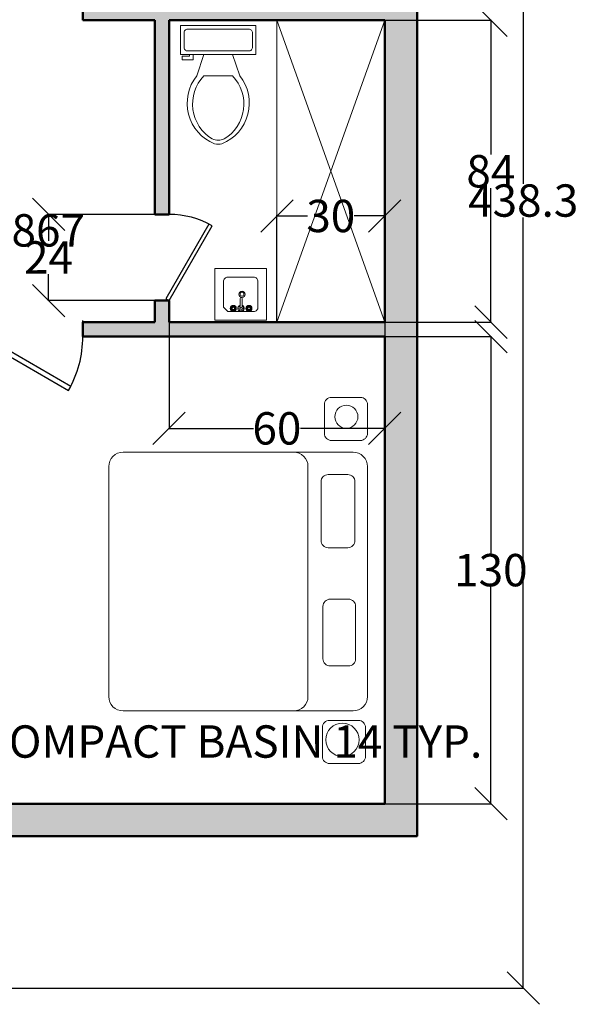
# Model space of a CAD drawing. Units: inches. Extents: x -9 to 615, y -420 to 89.
# Tile 4 of 6: x 460 to 615, y -389 to -115. Entities that reach past the tile are written whole.
import ezdxf

# ---------------------------------------------------------------- set-up
doc = ezdxf.new("R2010")
doc.units = ezdxf.units.IN
doc.header["$MEASUREMENT"] = 0
for name, color, linetype, lineweight in [('A-ANNO-DIMS', 2, 'Continuous', 18), ('A-DOOR', 4, 'Continuous', 25), ('A-FLOR-FIXT', 9, 'Continuous', 18), ('A-FURN', 8, 'Continuous', 18), ('A-WALL', 7, 'Continuous', 50)]:
    doc.layers.add(name, color=color, linetype=linetype, lineweight=lineweight)
doc.layers.add('A-WALL-PATT', color=251, linetype='Continuous', lineweight=13, true_color=0x636466)
doc.styles.get("Standard").update_dxf_attribs({"font": 'arial.ttf'})
doc.dimstyles.get("Standard").update_dxf_attribs({"dimtxt": 9, "dimasz": 9, "dimexe": 0.18, "dimexo": 0.0625, "dimgap": 0.09, "dimtad": 0, "dimtih": 1, "dimtoh": 1, "dimdec": 0, "dimzin": 0, "dimdsep": 46, "dimlunit": 4, "dimtxsty": 'Standard', "dimblk": 'OBLIQUE', "dimblk2": 'OBLIQUE', "dimcen": 0.09, "dimadec": 0, "dimazin": 0, "dimtfac": 1, "dimtdec": 0, "dimtofl": 0, "dimtmove": 0, "dimatfit": 3, "dimldrblk": 'OBLIQUE', "dimfxl": 1, "dimtolj": 1, "dimtzin": 0, "dimarcsym": 0})

# ---------------------------------------------------------------- blocks, each defined once
blk = doc.blocks.new('6 BED')
for p, q in [((-33.45, 25.64), (30.55, 25.64)), ((-37.45, 21.64), (-37.45, -23.43)), ((34.55, 21.64), (34.55, -19.64))]:
    blk.add_line(p, q)
for points in [[(-42.69, 42.2), (-50.69, 42.2, 0.414214), (-52.69, 40.2), (-52.69, 32.2, 0.414214), (-50.69, 30.2), (-42.69, 30.2, 0.414214), (-40.69, 32.2), (-40.69, 40.2, 0.414214)], [(-33.45, 42.2), (30.55, 42.2, -0.414214), (34.55, 38.2), (34.55, -25.8, -0.414214), (30.55, -29.8), (-33.45, -29.8, -0.414214), (-37.45, -25.8), (-37.45, 38.2, -0.414214)], [(39.19, 41.65), (47.19, 41.65, -0.414214), (49.19, 39.65), (49.19, 31.65, -0.414214), (47.19, 29.65), (39.19, 29.65, -0.414214), (37.19, 31.65), (37.19, 39.65, -0.414214)], [(-29.22, 38.71), (-12.85, 38.71, -0.414214), (-10.85, 36.71), (-10.85, 31.26, -0.414214), (-12.85, 29.26), (-29.22, 29.26, -0.414214), (-31.22, 31.26), (-31.22, 36.71, -0.414214)], [(5.45, 38.89), (20.03, 38.89, -0.414214), (22.03, 36.89), (22.03, 31.79, -0.414214), (20.03, 29.79), (5.45, 29.79, -0.414214), (3.45, 31.79), (3.45, 36.89, -0.414214)]]:
    blk.add_lwpolyline(points, format="xyb", close=True)
for centre, start, end in [((-33.45, 21.64), 90, 180), ((30.55, 21.64), 0, 90)]:
    blk.add_arc(centre, 4, start, end)
blk = doc.blocks.new('Toilet - top')
for p, q in [((9.5, -6), (9.5, -2)), ((-8, -8.5), (-8, -8)), ((-7, -8), (-7, -9.5)), ((-4, -8), (-6, -14)), ((4, -8), (6, -14)), ((-10, -8.5), (-8, -8.5)), ((-10, -9.5), (-10, -8.5)), ((-7, -9.5), (-10, -9.5)), ((4, -14), (-4, -14))]:
    blk.add_line(p, q)
blk.add_lwpolyline([(10.5, -8), (10.5, 0), (-10.5, 0), (-10.5, -8)], close=True)
for points in [[(-9.5, -2), (-9.5, -6)], [(8.5, -1), (-8.5, -1)], [(-8.5, -7), (8.5, -7)]]:
    blk.add_lwpolyline(points)
for centre, radius, start, end in [((-8.62, -1.88), 0.884, 81.8699, 188.1301), ((8.62, -1.88), 0.884, 351.8699, 98.1301), ((-8.62, -6.12), 0.884, 171.8699, 278.1301), ((8.62, -6.12), 0.884, 261.8699, 8.1301), ((3.52, -21.58), 12.17, 141.4691, 247.9714), ((4.2, -21.82), 11.33, 136.3677, 238.9468), ((-3.52, -21.58), 12.17, 292.0284, 38.5307), ((-4.2, -21.82), 11.33, 301.053, 43.6321), ((0, -27.88), 4, 245.7318, 294.2682), ((0, -29), 4, 254.8605, 285.1395)]:
    blk.add_arc(centre, radius, start, end)
blk = doc.blocks.new('*U12')
for p, q in [((0, 0), (0, -6)), ((40, 0), (40, -6))]:
    blk.add_line(p, q)
blk.add_lwpolyline([(0, 0), (34.64, 20), (35.52, 18.48), (0.87, -1.52)], close=True)
blk.add_arc((0, 0), 40, 0, 30)
blk = doc.blocks.new('*U13')
for p, q in [((0, 0), (0, 6)), ((40, 0), (40, 6))]:
    blk.add_line(p, q)
blk.add_lwpolyline([(0, 0), (34.64, -20), (35.52, -18.48), (0.87, 1.52)], close=True)
blk.add_arc((0, 0), 40, 330, 0)
blk = doc.blocks.new('Faucet - Bathroom top')
for p, q in [((-4.107, 0.125), (-4.375, 0.125)), ((-3.75, 0.4788), (-3.75, 0.75)), ((-3.5, 0.482), (-3.5, 0.75)), ((-3.1461, 0.125), (-2.875, 0.125)), ((3.143, 0.125), (2.875, 0.125)), ((3.5, 0.4788), (3.5, 0.75)), ((3.75, 0.482), (3.75, 0.75)), ((4.1039, 0.125), (4.375, 0.125)), ((-4.1039, -0.125), (-4.375, -0.125)), ((-3.75, -0.4821), (-3.75, -0.75)), ((-3.5, -0.4789), (-3.5, -0.75)), ((-3.143, -0.125), (-2.875, -0.125)), ((-0.5, -0.8639), (-0.5, -4.5)), ((0.5, -4.5), (0.5, -0.8631)), ((3.1461, -0.125), (2.875, -0.125)), ((3.5, -0.4821), (3.5, -0.75)), ((3.75, -0.4789), (3.75, -0.75)), ((4.107, -0.125), (4.375, -0.125))]:
    blk.add_line(p, q)
for centre, radius in [((-3.625, 0), 1.375), ((-4.625, 0), 0.2795), ((-3.625, 0), 0.5), ((-3.625, 1), 0.2795), ((-2.625, 0), 0.2795), ((0, 0), 0.5), ((3.625, 0), 1.375), ((2.625, 0), 0.2795), ((3.625, 0), 0.5), ((3.625, 1), 0.2795), ((4.625, 0), 0.2795), ((-3.625, -1), 0.2795), ((3.625, -1), 0.2795)]:
    blk.add_circle(centre, radius)
for centre, radius, start, end in [((-3.625, 0), 1, 105.2407, 164.2093), ((-3.625, 0), 1, 16.44125, 74.07887), ((0, 0), 1.5, 289.6514, 250.3603), ((0, 0), 1, 300.3431, 239.7554), ((3.625, 0), 1, 106.12, 164.0884), ((3.625, 0), 1, 16.23422, 73.90469), ((-3.625, 0), 1, 196.2342, 253.9047), ((-3.625, 0), 1, 286.12, 344.0884), ((0, -4.5), 0.5, 180, 0), ((3.625, 0), 1, 196.4413, 254.0789), ((3.625, 0), 1, 285.2407, 344.2093)]:
    blk.add_arc(centre, radius, start, end)
blk = doc.blocks.new('LAVATORY-COMPACT')
blk.add_lwpolyline([(14.42, 0), (14.42, 14.37), (0, 14.37), (0, 0)], close=True)
blk.add_lwpolyline([(12.02, 3.61), (12.02, 10.76, 0.414214), (10.82, 11.96), (3.61, 11.96, 0.414214), (2.4, 10.76), (2.4, 3.61), (3.61, 2.4), (10.82, 2.4, 0.414214)], format="xyb", close=True)
for centre, radius in [((7.57, 7.22), 0.886), ((7.57, 7.26), 0.547)]:
    blk.add_circle(centre, radius)
at = {"xscale": 0.6009252125773316, "yscale": 0.6009252125773316, "zscale": 0.6009252125773316, "rotation": 180}
blk.add_blockref('Faucet - Bathroom top', (7.32, 3.3), dxfattribs=at)
blk = doc.blocks.new('_Oblique')
at = {"color": 0, "linetype": 'ByBlock', "lineweight": -2}
blk.add_line((-0.5, -0.5), (0.5, 0.5), dxfattribs=at)
blk = doc.blocks.new('*D24')
at = {"layer": 'A-ANNO-DIMS', "color": 0, "lineweight": -2, "transparency": 16777216}
for p, q in [((419.63, -317.77), (419.63, -315.49)), ((419.63, -315.67), (434.05, -315.67)), ((434.05, -317.77), (434.05, -315.49)), ((434.05, -315.67), (443.05, -315.67))]:
    blk.add_line(p, q, dxfattribs=at)
at = {"layer": 'Defpoints', "color": 0, "transparency": 16777216}
for p in [(434.05, -315.67), (419.63, -317.84), (434.05, -317.84)]:
    blk.add_point(p, dxfattribs=at)
at = {"layer": 'A-ANNO-DIMS', "color": 0, "lineweight": -2, "transparency": 16777216, "xscale": 9, "yscale": 9, "zscale": 9, "rotation": 180}
blk.add_blockref('_Oblique', (419.63, -315.67), dxfattribs=at)
at = {"layer": 'A-ANNO-DIMS', "color": 0, "lineweight": -2, "transparency": 16777216, "xscale": 9, "yscale": 9, "zscale": 9}
blk.add_blockref('_Oblique', (434.05, -315.67), dxfattribs=at)
at = {"layer": 'A-ANNO-DIMS', "color": 0, "transparency": 16777216, "insert": (518.79, -315.67), "char_height": 9, "attachment_point": 5}
blk.add_mtext('\\A1;COMPACT BASIN 14 TYP.', dxfattribs=at)
blk = doc.blocks.new('*D42')
at = {"layer": 'A-ANNO-DIMS', "color": 0, "lineweight": -2, "transparency": 16777216}
for p, q in [((437.5, 54.02), (600.17, 54.02)), ((599.99, 54.02), (599.99, -160.45)), ((599.99, -384.29), (599.99, -169.82)), ((365.62, -384.29), (600.17, -384.29))]:
    blk.add_line(p, q, dxfattribs=at)
at = {"layer": 'Defpoints', "color": 0, "transparency": 16777216}
for p in [(437.44, 54.02), (599.99, 54.02), (365.56, -384.29)]:
    blk.add_point(p, dxfattribs=at)
at = {"layer": 'A-ANNO-DIMS', "color": 0, "lineweight": -2, "transparency": 16777216, "xscale": 9, "yscale": 9, "zscale": 9}
for p, rotation in [((599.99, 54.02), 90), ((599.99, -384.29), 270)]:
    blk.add_blockref('_Oblique', p, dxfattribs=dict(at, rotation=rotation))
at = {"layer": 'A-ANNO-DIMS', "color": 0, "transparency": 16777216, "insert": (599.99, -165.14), "char_height": 9, "attachment_point": 5}
blk.add_mtext('\\A1;438.3', dxfattribs=at)
blk = doc.blocks.new('*D58')
at = {"layer": 'A-ANNO-DIMS', "color": 0, "lineweight": -2, "transparency": 16777216}
for p, q in [((561.5, -114.98), (591.17, -114.98)), ((590.99, -114.98), (590.99, -152.3)), ((590.99, -198.98), (590.99, -161.67)), ((561.5, -198.98), (591.17, -198.98))]:
    blk.add_line(p, q, dxfattribs=at)
at = {"layer": 'Defpoints', "color": 0, "transparency": 16777216}
for p in [(561.44, -114.98), (561.44, -198.98), (590.99, -198.98)]:
    blk.add_point(p, dxfattribs=at)
at = {"layer": 'A-ANNO-DIMS', "color": 0, "lineweight": -2, "transparency": 16777216, "xscale": 9, "yscale": 9, "zscale": 9}
for p, rotation in [((590.99, -114.98), 90), ((590.99, -198.98), 270)]:
    blk.add_blockref('_Oblique', p, dxfattribs=dict(at, rotation=rotation))
at = {"layer": 'A-ANNO-DIMS', "color": 0, "transparency": 16777216, "insert": (590.99, -156.98), "char_height": 9, "attachment_point": 5}
blk.add_mtext('\\A1;84', dxfattribs=at)
blk = doc.blocks.new('*D59')
at = {"layer": 'A-ANNO-DIMS', "color": 0, "lineweight": -2, "transparency": 16777216}
for p, q in [((561.5, -202.98), (591.17, -202.98)), ((590.99, -202.98), (590.99, -263.29)), ((590.99, -332.98), (590.99, -272.67)), ((561.5, -332.98), (591.17, -332.98))]:
    blk.add_line(p, q, dxfattribs=at)
at = {"layer": 'Defpoints', "color": 0, "transparency": 16777216}
for p in [(561.44, -202.98), (561.44, -332.98), (590.99, -332.98)]:
    blk.add_point(p, dxfattribs=at)
at = {"layer": 'A-ANNO-DIMS', "color": 0, "lineweight": -2, "transparency": 16777216, "xscale": 9, "yscale": 9, "zscale": 9}
for p, rotation in [((590.99, -202.98), 90), ((590.99, -332.98), 270)]:
    blk.add_blockref('_Oblique', p, dxfattribs=dict(at, rotation=rotation))
at = {"layer": 'A-ANNO-DIMS', "color": 0, "transparency": 16777216, "insert": (590.99, -267.98), "char_height": 9, "attachment_point": 5}
blk.add_mtext('\\A1;130', dxfattribs=at)
blk = doc.blocks.new('*D61')
at = {"layer": 'A-ANNO-DIMS', "color": 0, "lineweight": -2, "transparency": 16777216}
for p, q in [((501.44, -199.04), (501.44, -228.71)), ((561.44, -199.04), (561.44, -228.71)), ((501.44, -228.53), (524.89, -228.53)), ((561.44, -228.53), (537.98, -228.53))]:
    blk.add_line(p, q, dxfattribs=at)
at = {"layer": 'Defpoints', "color": 0, "transparency": 16777216}
for p in [(501.44, -198.98), (561.44, -198.98), (501.44, -228.53)]:
    blk.add_point(p, dxfattribs=at)
at = {"layer": 'A-ANNO-DIMS', "color": 0, "lineweight": -2, "transparency": 16777216, "xscale": 9, "yscale": 9, "zscale": 9, "rotation": 180}
blk.add_blockref('_Oblique', (501.44, -228.53), dxfattribs=at)
at = {"layer": 'A-ANNO-DIMS', "color": 0, "lineweight": -2, "transparency": 16777216, "xscale": 9, "yscale": 9, "zscale": 9}
blk.add_blockref('_Oblique', (561.44, -228.53), dxfattribs=at)
at = {"layer": 'A-ANNO-DIMS', "color": 0, "transparency": 16777216, "insert": (531.44, -228.53), "char_height": 9, "attachment_point": 5}
blk.add_mtext('\\A1;60', dxfattribs=at)
blk = doc.blocks.new('*D83')
at = {"layer": 'A-ANNO-DIMS', "color": 0, "lineweight": -2, "transparency": 16777216}
for p, q in [((407.57, -202.92), (407.57, -173.25)), ((407.57, -173.43), (431.44, -173.43)), ((431.44, -202.92), (431.44, -173.25)), ((431.44, -173.43), (440.44, -173.43))]:
    blk.add_line(p, q, dxfattribs=at)
at = {"layer": 'Defpoints', "color": 0, "transparency": 16777216}
for p in [(431.44, -173.43), (407.57, -202.98), (431.44, -202.98)]:
    blk.add_point(p, dxfattribs=at)
at = {"layer": 'A-ANNO-DIMS', "color": 0, "lineweight": -2, "transparency": 16777216, "xscale": 9, "yscale": 9, "zscale": 9}
for p, rotation in [((407.57, -173.43), 179.9957313398861), ((431.44, -173.43), 359.995731339886)]:
    blk.add_blockref('_Oblique', p, dxfattribs=dict(at, rotation=rotation))
at = {"layer": 'A-ANNO-DIMS', "color": 0, "transparency": 16777216, "insert": (459.29, -173.43), "char_height": 9, "attachment_point": 5}
blk.add_mtext('\\A1;23.867', dxfattribs=at)
blk = doc.blocks.new('*D84')
at = {"layer": 'A-ANNO-DIMS', "color": 0, "lineweight": -2, "transparency": 16777216}
for p, q in [((497.38, -168.98), (467.71, -168.98)), ((467.89, -168.98), (467.89, -176.37)), ((467.89, -192.98), (467.89, -185.59)), ((497.38, -192.98), (467.71, -192.98))]:
    blk.add_line(p, q, dxfattribs=at)
at = {"layer": 'Defpoints', "color": 0, "transparency": 16777216}
for p in [(467.89, -168.98), (497.44, -168.98), (497.44, -192.98)]:
    blk.add_point(p, dxfattribs=at)
at = {"layer": 'A-ANNO-DIMS', "color": 0, "lineweight": -2, "transparency": 16777216, "xscale": 9, "yscale": 9, "zscale": 9}
for p, rotation in [((467.89, -168.98), 90), ((467.89, -192.98), 270)]:
    blk.add_blockref('_Oblique', p, dxfattribs=dict(at, rotation=rotation))
at = {"layer": 'A-ANNO-DIMS', "color": 0, "transparency": 16777216, "insert": (467.89, -180.98), "char_height": 9, "attachment_point": 5}
blk.add_mtext('\\A1;24', dxfattribs=at)
blk = doc.blocks.new('*D85')
at = {"layer": 'A-ANNO-DIMS', "color": 0, "lineweight": -2, "transparency": 16777216}
for p, q in [((531.44, -198.92), (531.44, -169.25)), ((531.44, -169.43), (539.92, -169.43)), ((561.44, -169.43), (552.96, -169.43)), ((561.44, -198.92), (561.44, -169.25))]:
    blk.add_line(p, q, dxfattribs=at)
at = {"layer": 'Defpoints', "color": 0, "transparency": 16777216}
for p in [(561.44, -169.43), (531.44, -198.98), (561.44, -198.98)]:
    blk.add_point(p, dxfattribs=at)
at = {"layer": 'A-ANNO-DIMS', "color": 0, "lineweight": -2, "transparency": 16777216, "xscale": 9, "yscale": 9, "zscale": 9, "rotation": 180}
blk.add_blockref('_Oblique', (531.44, -169.43), dxfattribs=at)
at = {"layer": 'A-ANNO-DIMS', "color": 0, "lineweight": -2, "transparency": 16777216, "xscale": 9, "yscale": 9, "zscale": 9}
blk.add_blockref('_Oblique', (561.44, -169.43), dxfattribs=at)
at = {"layer": 'A-ANNO-DIMS', "color": 0, "transparency": 16777216, "insert": (546.44, -169.43), "char_height": 9, "attachment_point": 5}
blk.add_mtext('\\A1;30', dxfattribs=at)

msp = doc.modelspace()

# ---------------------------------------------------------------- hatches: boundary and pattern name
at = {"layer": 'A-WALL-PATT'}
h = msp.add_hatch(color=256, dxfattribs=at)
h.dxf.hatch_style = 1
h.paths.add_polyline_path([(570.4378, 18.0183), (437.4378, 18.0183), (437.4378, -14.9817), (437.4378, -110.9817), (385.4378, -110.9817), (385.4378, -114.9817), (385.4378, -120.9817), (389.4378, -120.9817), (389.4378, -114.9817), (437.4378, -114.9817), (447.4378, -114.9817), (447.4378, -110.9817), (441.4378, -110.9817), (441.4378, 9.0183), (561.4378, 9.0183), (561.4378, -110.9817), (477.4378, -110.9817), (477.4378, -114.9817), (497.4378, -114.9817), (497.4378, -168.9817), (501.4378, -168.9817), (501.4378, -114.9817), (561.4378, -114.9817), (561.4378, -198.9817), (531.4378, -198.9817), (501.4378, -198.9817), (501.4378, -192.9817), (497.4378, -192.9817), (497.4378, -198.9817), (477.4378, -198.9817), (477.4378, -202.9817), (561.4378, -202.9817), (561.4378, -332.9817), (441.4378, -332.9817), (441.4378, -202.9817), (447.4378, -202.9817), (447.4378, -198.9817), (437.4378, -198.9817), (431.4378, -198.9817), (431.4378, -202.9817), (437.4378, -202.9817), (437.4378, -256.9817), (389.4378, -256.9817), (389.4378, -202.9799), (407.5704, -202.9799), (407.4511, -198.9817), (389.4378, -198.9817), (385.4378, -198.9817), (385.4378, -302.9817), (389.4378, -302.9817), (389.4378, -260.9817), (437.4378, -260.9817), (437.4378, -332.9817), (389.4378, -332.9817), (389.4378, -326.9817), (385.4378, -326.9817), (385.4378, -332.9817), (352.4378, -332.9817), (352.4378, -341.9817), (570.4378, -341.9817)])

# ---------------------------------------------------------------- linework, layer by layer
at = {"layer": 'A-FLOR-FIXT'}
for p, q in [((531.4378, -114.9817), (561.4378, -198.9817)), ((561.4378, -114.9817), (531.4378, -198.9817))]:
    msp.add_line(p, q, dxfattribs=at)
msp.add_lwpolyline([(561.4378, -114.9817), (531.4378, -114.9817), (531.4378, -198.9817), (561.4378, -198.9817)], close=True, dxfattribs=at)
at = {"layer": 'A-FURN'}
for centre, radius in [((550.7687, -225.2963), 3.2166), ((549.6687, -315.195), 4.6429)]:
    msp.add_circle(centre, radius, dxfattribs=at)
at = {"layer": 'A-WALL'}
for p, q in [((477.4378, -110.9817), (477.4378, -114.9817)), ((477.4378, -114.9817), (497.4378, -114.9817)), ((497.4378, -114.9817), (497.4378, -168.9817)), ((501.4378, -114.9817), (501.4378, -168.9817)), ((501.4378, -114.9817), (561.4378, -114.9817)), ((561.4378, -114.9817), (561.4378, -198.9817)), ((497.4378, -168.9817), (501.4378, -168.9817)), ((497.4378, -192.9817), (501.4378, -192.9817)), ((497.4378, -192.9817), (497.4378, -198.9817)), ((501.4378, -192.9817), (501.4378, -198.9817)), ((477.4378, -202.9817), (477.4378, -198.9817)), ((477.4378, -198.9817), (497.4378, -198.9817)), ((501.4378, -198.9817), (561.4378, -198.9817)), ((477.4378, -202.9817), (561.4378, -202.9817)), ((561.4378, -202.9817), (561.4378, -332.9817)), ((561.4378, -332.9817), (441.4378, -332.9817))]:
    msp.add_line(p, q, dxfattribs=at)
msp.add_lwpolyline([(437.4378, 18.0183), (570.4378, 18.0183), (570.4378, -341.9817), (352.4378, -341.9817)], dxfattribs=at)

# ---------------------------------------------------------------- block references
at = {"layer": 'A-DOOR', "xscale": 0.75, "yscale": 0.75, "zscale": 0.75}
for name, p in [('*U12', (447.4378, -110.4817)), ('*U13', (447.4378, -202.9817))]:
    msp.add_blockref(name, p, dxfattribs=at)
at = {"layer": 'A-DOOR', "xscale": 0.6, "yscale": 0.6, "zscale": 0.6, "rotation": 90}
msp.add_blockref('*U13', (501.4378, -192.9817), dxfattribs=at)
at = {"layer": 'A-FLOR-FIXT'}
for name, p in [('Toilet - top', (515.1161, -116.4764)), ('LAVATORY-COMPACT', (514.161, -198.441))]:
    msp.add_blockref(name, p, dxfattribs=at)
at = {"layer": 'A-FURN', "rotation": 270}
msp.add_blockref('6 BED', (514.4569, -272.605), dxfattribs=at)

# ---------------------------------------------------------------- dimensions: what is measured, and where the dimension line sits
at = {"layer": 'A-ANNO-DIMS'}
for base, p1, p2, angle, override, picture, middle in [((599.9878, 54.0183), (365.5581, -384.2897), (437.4378, 54.0183), 90, {"dimdec": 1, "dimlfac": 1, "dimrnd": 0, "dimzin": 0, "dimdsep": 46, "dimlunit": 2}, '*D42', (599.9878, -165.1357)), ((590.9878, -198.9817), (561.4378, -114.9817), (561.4378, -198.9817), 270, {"dimdec": 0, "dimlfac": 1, "dimrnd": 0, "dimzin": 0, "dimdsep": 46, "dimlunit": 2}, '*D58', (590.9878, -156.9817)), ((467.8878, -168.9817), (497.4378, -192.9817), (497.4378, -168.9817), 90, {"dimdec": 0, "dimlfac": 1, "dimrnd": 0, "dimzin": 0, "dimdsep": 46, "dimlunit": 2}, '*D84', (467.8878, -180.9817)), ((431.44, -173.4317), (407.5704, -202.9799), (431.4378, -202.9817), 359.995731, {"dimdec": 3, "dimlfac": 1, "dimrnd": 0, "dimzin": 0, "dimdsep": 46, "dimlunit": 2}, '*D83', (459.2882, -173.4324)), ((501.4378, -228.5317), (561.4378, -198.9817), (501.4378, -198.9817), 180, {"dimdec": 0, "dimlfac": 1, "dimrnd": 0, "dimzin": 0, "dimdsep": 46, "dimlunit": 2}, '*D61', (531.4378, -228.5317)), ((590.9878, -332.9817), (561.4378, -202.9817), (561.4378, -332.9817), 270, {"dimdec": 0, "dimlfac": 1, "dimrnd": 0, "dimzin": 0, "dimdsep": 46, "dimlunit": 2}, '*D59', (590.9878, -267.9817))]:
    dim = msp.add_linear_dim(base=base, p1=p1, p2=p2, angle=angle, dimstyle='Standard', override=override, dxfattribs=at)
    dim.commit()
    dim.dimension.update_dxf_attribs({"geometry": picture, "text_midpoint": middle})
dim = msp.add_linear_dim(base=(561.4378, -169.4317), p1=(531.4378, -198.9817), p2=(561.4378, -198.9817), dimstyle='Standard', override={"dimdec": 0, "dimlfac": 1, "dimrnd": 0, "dimzin": 0, "dimdsep": 46, "dimlunit": 2}, dxfattribs=at)
dim.commit()
dim.dimension.update_dxf_attribs({"geometry": '*D85', "text_midpoint": (546.4378, -169.4317)})
dim = msp.add_linear_dim(base=(434.0539, -315.6735), p1=(419.6317, -317.8368), p2=(434.0539, -317.8368), text='COMPACT BASIN <> TYP.', dimstyle='Standard', override={"dimdec": 0, "dimlfac": 1, "dimrnd": 0, "dimzin": 0, "dimdsep": 46, "dimlunit": 2}, dxfattribs=at)
dim.commit()
dim.dimension.update_dxf_attribs({"geometry": '*D24', "text_midpoint": (518.7875, -315.6735)})

doc.saveas('drawing.dxf')
